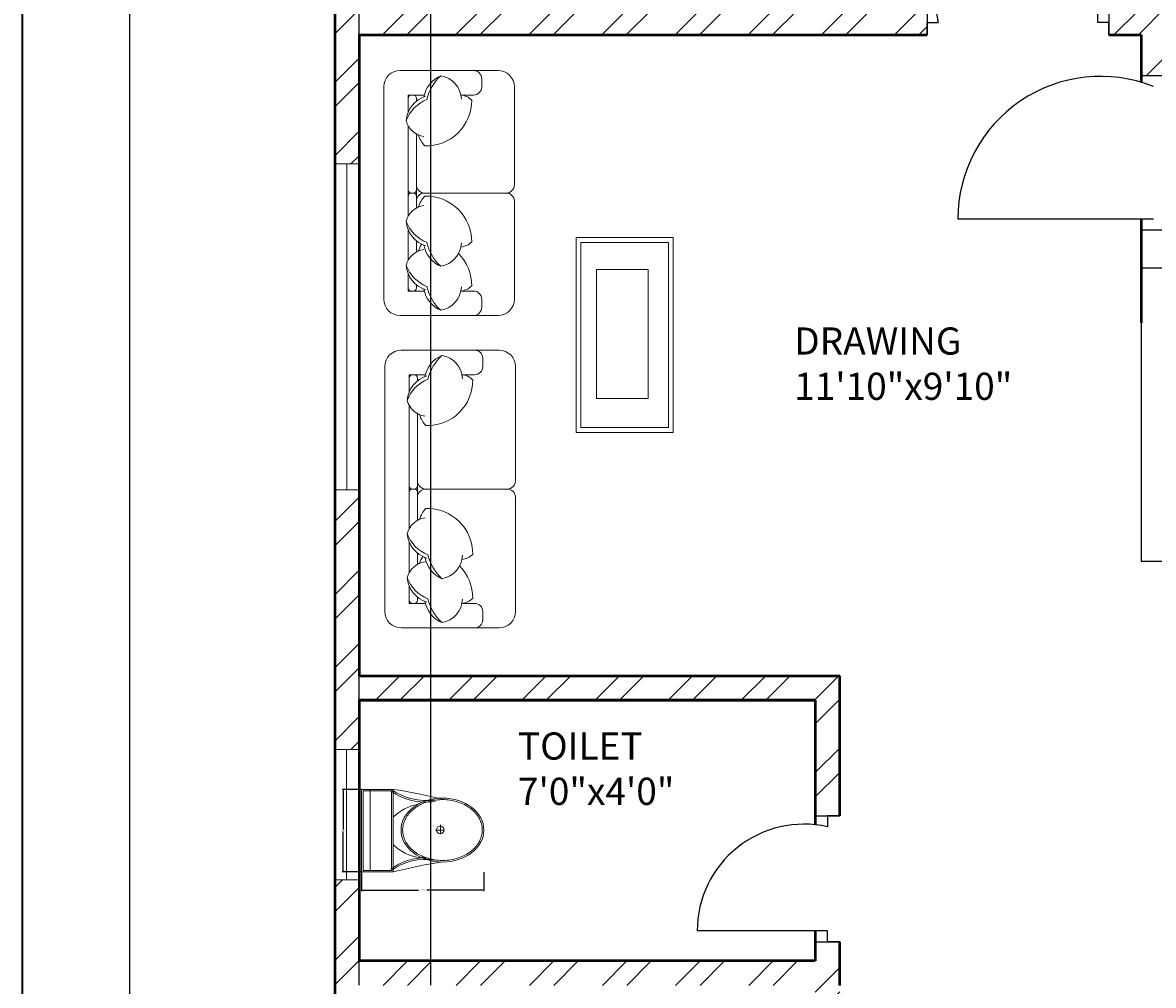
# Model space of a CAD drawing. Units: inches. Extents: x 2129 to 2642, y 1542 to 2414.
# Tile 5 of 9: x 2129 to 2338, y 2007 to 2184. Entities that reach past the tile are written whole.
import ezdxf

# ---------------------------------------------------------------- set-up
doc = ezdxf.new("R2010")
doc.units = ezdxf.units.IN
for name, color, linetype, lineweight in [('A-ANNO-DIMS', 2, 'Continuous', 18), ('A-ANNO-TTLB', 7, 'Continuous', 35), ('A-AREA-IDEN', 7, 'Continuous', 18), ('A-DOOR', 3, 'Continuous', 25), ('A-FLOR-EVTR', 141, 'Continuous', 25), ('A-FLOR-FIXT', 9, 'Continuous', 18), ('A-FURN', 8, 'Continuous', 18), ('A-GLAZ', 4, 'Continuous', 18), ('A-WALL', 7, 'Continuous', 50), ('A-WALL-PATT', 252, 'Continuous', 13)]:
    doc.layers.add(name, color=color, linetype=linetype, lineweight=lineweight)
doc.styles.get("Standard").update_dxf_attribs({"font": 'arial.ttf'})
doc.dimstyles.get("Standard").update_dxf_attribs({"dimtxt": 0.18, "dimasz": 0.18, "dimexe": 0.18, "dimexo": 0.0625, "dimgap": 0.09, "dimtad": 0, "dimtih": 1, "dimtoh": 1, "dimdec": 4, "dimzin": 0, "dimdsep": 46, "dimtxsty": 'Standard', "dimcen": 0.09, "dimadec": 0, "dimazin": 0, "dimtfac": 1, "dimtdec": 4, "dimtofl": 0, "dimtmove": 0, "dimatfit": 3, "dimfxl": 1, "dimtolj": 1, "dimtzin": 0, "dimarcsym": 0})

# ---------------------------------------------------------------- blocks, each defined once
blk = doc.blocks.new('A$C31115884')
for p, q in [((257.5, 466.4), (257.5, 523.2)), ((283.1, 497.7), (223.4, 497.7)), ((0, 200), (0, 0)), ((520, 200), (0, 200)), ((10, 190), (10, 10)), ((510, 190), (10, 190)), ((510, 10), (510, 190)), ((520, 0), (520, 200)), ((510, 54.5), (0, 54.5)), ((10, 10), (510, 10)), ((0, 0), (520, 0))]:
    blk.add_line(p, q)
blk.add_circle((255.6, 496.4), 23.6)
for centre, radius, start, end in [((2777.7, -204.6), 2807, 165.4549, 171.71327), ((3237, 905), 2807, 188.28673, 194.5451), ((-294.5, 403.3), 364.7, 324.20913, 9.34987), ((-294.5, 403.3), 374.7, 324.20913, 9.34987), ((805.8, 403.3), 364.7, 170.65013, 215.79087), ((139.5, 406.2), 293.5, 315.84364, 2.65635), ((805.8, 403.3), 374.7, 179.20365, 215.79087), ((383.6, 406.2), 293.5, 190.27735, 224.15636)]:
    blk.add_arc(centre, radius, start, end)
blk.add_ellipse((256.2, 509.9), major_axis=(0, -260.7), ratio=0.772727)
blk.add_open_spline([(256.2, 259.2), (263.1, 259.2), (270, 259.7), (287.8, 262.3), (298.7, 265.1), (319.9, 273.1), (330.2, 278.4), (350.1, 291.1), (359.7, 298.7), (377.7, 315.9), (386.2, 325.5), (401.7, 346.6), (408.8, 358.1), (421.3, 382.5), (426.8, 395.5), (435.9, 422.4), (439.5, 436.4), (444.8, 465.1), (446.5, 479.7), (447.9, 509.2), (447.6, 524), (445, 553.3), (442.7, 567.8), (436.3, 596), (432.1, 609.7), (421.9, 636), (416, 648.6), (402.5, 672.1), (395, 683), (378.6, 703), (369.8, 712.1), (351.1, 728), (341.3, 734.8), (320.9, 746.2), (310.4, 750.7), (288.9, 757.3), (278, 759.4), (256, 761), (245, 760.6), (223.1, 757.2), (212.3, 754.3), (191.1, 746.1), (180.8, 740.7), (160.9, 727.8), (151.4, 720.1), (133.5, 702.7), (125.1, 693), (109.6, 671.7), (102.6, 660.2), (90.2, 635.7), (84.9, 622.7), (76, 595.6), (72.4, 581.6), (67.2, 552.9), (65.6, 538.2), (64.4, 508.8), (64.8, 494), (67.5, 464.7), (69.9, 450.2), (76.6, 422), (80.8, 408.3), (91.1, 382.2), (97.2, 369.7), (110.8, 346.3), (118.4, 335.4), (134.8, 315.6), (143.7, 306.7), (162.4, 290.9), (172.3, 284.2), (192.8, 273), (203.3, 268.6), (224.8, 262.2), (235.8, 260.2), (249.9, 259.3), (253, 259.2), (256.2, 259.2)], degree=3, knots=[0, 0, 0, 0, 0.110105, 0.110105, 0.285049, 0.285049, 0.459994, 0.459994, 0.634938, 0.634938, 0.809882, 0.809882, 0.984827, 0.984827, 1.159771, 1.159771, 1.334715, 1.334715, 1.50966, 1.50966, 1.684604, 1.684604, 1.859549, 1.859549, 2.034493, 2.034493, 2.209437, 2.209437, 2.384382, 2.384382, 2.559326, 2.559326, 2.73427, 2.73427, 2.909215, 2.909215, 3.084159, 3.084159, 3.259103, 3.259103, 3.434048, 3.434048, 3.608992, 3.608992, 3.783936, 3.783936, 3.958881, 3.958881, 4.133825, 4.133825, 4.30877, 4.30877, 4.483714, 4.483714, 4.658658, 4.658658, 4.833603, 4.833603, 5.008547, 5.008547, 5.183491, 5.183491, 5.358436, 5.358436, 5.53338, 5.53338, 5.708324, 5.708324, 5.883269, 5.883269, 6.058213, 6.058213, 6.233158, 6.233158, 6.283185, 6.283185, 6.283185, 6.283185])
blk = doc.blocks.new('TABLE-COFFEE')
for points in [[(0, 35.92), (17.84, 35.92), (17.84, 0), (0, 0)], [(0.86, 34.99), (17.01, 34.99), (17.01, 0.93), (0.86, 0.93)], [(3.74, 30.05), (13.25, 30.05), (13.25, 6.3), (3.74, 6.3)]]:
    blk.add_lwpolyline(points, close=True)
blk = doc.blocks.new('WIN-60-B')
for p, q in [((4.5, 60), (0, 60)), ((0, 60), (2.25, 60)), ((2.25, 60), (2.25, 0)), ((2.25, 0), (0, 0)), ((0, 0), (4.5, 0))]:
    blk.add_line(p, q)
blk = doc.blocks.new('*D20')
at = {"layer": 'A-ANNO-DIMS', "color": 0, "lineweight": -2, "transparency": 16777216}
for p, q in [((2191.83, 2028.04), (2191.83, 2024.55)), ((2214.37, 2028.04), (2214.37, 2024.55)), ((2192.01, 2024.73), (2202.33, 2024.73)), ((2214.19, 2024.73), (2203.88, 2024.73))]:
    blk.add_line(p, q, dxfattribs=at)
at = {"layer": 'A-ANNO-DIMS', "color": 0, "transparency": 16777216}
for points in [[(2192.01, 2024.76), (2192.01, 2024.7), (2191.83, 2024.73)], [(2214.19, 2024.76), (2214.19, 2024.7), (2214.37, 2024.73)]]:
    blk.add_solid(points, dxfattribs=at)
at = {"layer": 'Defpoints', "color": 0, "transparency": 16777216}
for p in [(2191.83, 2028.11), (2214.37, 2028.11), (2214.37, 2024.73)]:
    blk.add_point(p, dxfattribs=at)
at = {"layer": 'A-ANNO-DIMS', "color": 0, "transparency": 16777216, "insert": (2203.1, 2024.73), "char_height": 0.18, "attachment_point": 5}
blk.add_mtext('\\A1;WC 23 TYP.', dxfattribs=at)
blk = doc.blocks.new('*D21')
at = {"layer": 'A-ANNO-DIMS', "color": 0, "lineweight": -2, "transparency": 16777216}
for p, q in [((2191.77, 2043.31), (2188.27, 2043.31)), ((2188.45, 2043.13), (2188.45, 2035.89)), ((2188.45, 2028.29), (2188.45, 2035.53)), ((2191.77, 2028.11), (2188.27, 2028.11))]:
    blk.add_line(p, q, dxfattribs=at)
at = {"layer": 'A-ANNO-DIMS', "color": 0, "transparency": 16777216}
for points in [[(2188.42, 2043.13), (2188.48, 2043.13), (2188.45, 2043.31)], [(2188.42, 2028.29), (2188.48, 2028.29), (2188.45, 2028.11)]]:
    blk.add_solid(points, dxfattribs=at)
at = {"layer": 'Defpoints', "color": 0, "transparency": 16777216}
for p in [(2191.83, 2043.31), (2188.45, 2028.11), (2191.83, 2028.11)]:
    blk.add_point(p, dxfattribs=at)
at = {"layer": 'A-ANNO-DIMS', "color": 0, "transparency": 16777216, "insert": (2188.45, 2035.71), "char_height": 0.18, "attachment_point": 5}
blk.add_mtext('\\A1;15 TYP.', dxfattribs=at)
blk = doc.blocks.new('*D35')
at = {"layer": 'A-ANNO-DIMS', "color": 0, "lineweight": -2, "transparency": 16777216}
for p, q in [((2186.84, 2340.22), (2148.97, 2340.22)), ((2149.15, 2340.04), (2149.15, 2003.15)), ((2149.15, 1665.9), (2149.15, 2002.79)), ((2186.84, 1665.72), (2148.97, 1665.72))]:
    blk.add_line(p, q, dxfattribs=at)
at = {"layer": 'A-ANNO-DIMS', "color": 0, "transparency": 16777216}
for points in [[(2149.12, 2340.04), (2149.18, 2340.04), (2149.15, 2340.22)], [(2149.12, 1665.9), (2149.18, 1665.9), (2149.15, 1665.72)]]:
    blk.add_solid(points, dxfattribs=at)
at = {"layer": 'Defpoints', "color": 0, "transparency": 16777216}
for p in [(2149.15, 2340.22), (2186.9, 2340.22), (2186.9, 1665.72)]:
    blk.add_point(p, dxfattribs=at)
at = {"layer": 'A-ANNO-DIMS', "color": 0, "transparency": 16777216, "insert": (2149.15, 2002.97), "char_height": 0.18, "attachment_point": 5}
blk.add_mtext('\\A1;674.5', dxfattribs=at)
blk = doc.blocks.new('*D48')
at = {"layer": 'A-ANNO-DIMS', "color": 0, "lineweight": -2, "transparency": 16777216}
for p, q in [((2191.4, 2007.28), (2191.4, 2378.15)), ((2191.58, 2377.97), (2197.54, 2377.97)), ((2204.41, 2377.97), (2198.45, 2377.97)), ((2204.59, 2007.28), (2204.59, 2378.15))]:
    blk.add_line(p, q, dxfattribs=at)
at = {"layer": 'A-ANNO-DIMS', "color": 0, "transparency": 16777216}
for points in [[(2191.58, 2378), (2191.58, 2377.94), (2191.4, 2377.97)], [(2204.41, 2378), (2204.41, 2377.94), (2204.59, 2377.97)]]:
    blk.add_solid(points, dxfattribs=at)
at = {"layer": 'Defpoints', "color": 0, "transparency": 16777216}
for p in [(2204.59, 2377.97), (2191.4, 2007.22), (2204.59, 2007.22)]:
    blk.add_point(p, dxfattribs=at)
at = {"layer": 'A-ANNO-DIMS', "color": 0, "transparency": 16777216, "insert": (2198, 2377.97), "char_height": 0.18, "attachment_point": 5}
blk.add_mtext('\\A1;13.186', dxfattribs=at)

msp = doc.modelspace()

# ---------------------------------------------------------------- hatches: boundary and pattern name
at = {"layer": 'A-WALL-PATT'}
h = msp.add_hatch(dxfattribs=at)
h.set_pattern_fill('ANSI32', color=256)
h.paths.add_polyline_path([(2306.2606, 2305.9717), (2306.2606, 2308.2217), (2276.3515, 2308.2217), (2276.3515, 2303.7217), (2306.2606, 2303.7217)])
h.paths.add_polyline_path([(2216.3515, 2305.9717), (2216.3515, 2308.2217), (2186.9043, 2308.2217), (2186.9043, 2278.1696), (2191.4043, 2278.1696), (2191.4043, 2303.7217), (2216.3515, 2303.7217)])
h.paths.add_polyline_path([(2339.9043, 2335.7217), (2362.1938, 2335.7217), (2362.1938, 2340.2217), (2335.4043, 2340.2217), (2335.4043, 2308.2217), (2329.3487, 2308.2217), (2329.3487, 2305.9717), (2329.3487, 2303.7217), (2335.4043, 2303.7217), (2335.4043, 2186.7217), (2329.4345, 2186.7217), (2329.4345, 2182.2217), (2335.4043, 2182.2217), (2335.4043, 2174.7178), (2339.9043, 2174.7178), (2339.9043, 2182.2217), (2339.9043, 2303.7217)])
h.paths.add_polyline_path([(2440.4043, 2340.2217), (2411.654, 2340.2217), (2411.654, 2335.7217), (2435.9043, 2335.7217), (2435.9043, 2303.7217), (2435.9043, 2182.2217), (2435.9043, 2174.1935), (2438.1543, 2174.1935), (2440.4043, 2174.1935), (2440.4043, 2182.2217), (2444.653, 2182.2217), (2444.653, 2184.4717), (2444.653, 2186.7217), (2440.4043, 2186.7217), (2440.4043, 2303.7217), (2445.8547, 2303.7217), (2445.8547, 2308.2217), (2440.4043, 2308.2217)])
h.paths.add_polyline_path([(2498.2381, 2308.2217), (2470.3901, 2308.2217), (2470.3901, 2303.7217), (2498.2381, 2303.7217), (2498.2381, 2305.9717)])
h.paths.add_polyline_path([(2588.9043, 2308.2217), (2586.9043, 2308.2217), (2558.2381, 2308.2217), (2558.2381, 2303.7217), (2584.4043, 2303.7217), (2584.4043, 2279.1087), (2588.9043, 2279.1087)])
h.paths.add_polyline_path([(2588.9043, 2219.1087), (2584.4043, 2219.1087), (2584.4043, 2186.7217), (2478.0667, 2186.7217), (2478.0667, 2182.2217), (2584.4043, 2182.2217), (2584.4043, 2157.7883), (2588.9043, 2157.7883)])
h.paths.add_polyline_path([(2588.9043, 2097.7883), (2584.6063, 2097.7883), (2584.6063, 2075.5462, -0.09241561), (2584.4043, 2074.4627), (2584.4043, 2064.2217), (2495.9043, 2064.2217), (2495.9043, 2040.4611), (2500.4043, 2040.4611), (2500.4043, 2059.7217), (2584.4043, 2059.7217), (2584.4043, 2052.2164), (2588.9043, 2052.2164)])
h.paths.add_polyline_path([(2588.9043, 2028.2164), (2584.4043, 2028.2164), (2584.4043, 2011.7217), (2500.4043, 2011.7217), (2500.4043, 2015.243), (2498.1543, 2015.243), (2495.9043, 2015.243), (2495.9043, 2007.2217), (2495.9043, 2003.7597), (2500.4043, 2003.7597), (2500.4043, 2007.2217), (2584.4043, 2007.2217), (2584.4043, 1992.1997), (2588.9043, 1992.1997)])
h.paths.add_polyline_path([(2588.9043, 1956.1997), (2584.4043, 1956.1997), (2584.4043, 1941.2217), (2500.4043, 1941.2217), (2500.4043, 1985.1493), (2498.1543, 1985.1493), (2495.9043, 1985.1493), (2495.9043, 1941.2217), (2435.9043, 1941.2217), (2435.9043, 1930.3963), (2440.4043, 1930.3963), (2440.4043, 1936.7217), (2584.4043, 1936.7217), (2584.4043, 1909.8406), (2588.9043, 1909.8406)])
h.paths.add_polyline_path([(2588.9043, 1849.8406), (2584.4043, 1849.8406), (2584.4043, 1801.3526), (2588.9043, 1801.3526)])
h.paths.add_polyline_path([(2584.4043, 1828.7217), (2495.9043, 1828.7217), (2440.4043, 1828.7217), (2440.4043, 1905.2159), (2438.1543, 1905.2159), (2435.9043, 1905.2159), (2435.9043, 1828.7217), (2428.9101, 1828.7217), (2428.9101, 1824.2217), (2584.4043, 1824.2217)])
h.paths.add_polyline_path([(2588.9043, 1741.3526), (2584.4043, 1741.3526), (2584.4043, 1704.2217), (2468.3173, 1704.2217), (2468.3173, 1701.9717), (2468.3173, 1699.7217), (2588.9043, 1699.7217)])
h.paths.add_polyline_path([(2442.4043, 1761.7217), (2435.0216, 1761.7217), (2435.0216, 1757.2217), (2437.9043, 1757.2217), (2437.9043, 1665.7217), (2442.4043, 1665.7217), (2442.4043, 1667.7217), (2442.4043, 1699.7217), (2446.6907, 1699.7217), (2446.6907, 1701.9717), (2446.6907, 1704.2217), (2442.4043, 1704.2217)])
h.paths.add_polyline_path([(2390.4043, 1757.2217), (2410.8996, 1757.2217), (2410.8996, 1761.7217), (2360.1741, 1761.7217), (2360.1741, 1759.4717), (2360.1741, 1757.2217), (2385.9043, 1757.2217), (2385.9043, 1674.8326), (2390.4043, 1674.8326)])
h.paths.add_polyline_path([(2337.9043, 1757.2217), (2340.3592, 1757.2217), (2340.3592, 1759.4717), (2340.3592, 1761.7217), (2333.4043, 1761.7217), (2333.4043, 1704.2217), (2327.381, 1704.2217), (2327.381, 1701.9717), (2327.381, 1699.7217), (2333.4043, 1699.7217), (2333.4043, 1665.7217), (2337.9043, 1665.7217)])
h.paths.add_polyline_path([(2191.4043, 1743.4804), (2186.9043, 1743.4804), (2186.9043, 1699.7217), (2188.9043, 1699.7217), (2191.4043, 1699.7217), (2306.5617, 1699.7217), (2306.5617, 1704.2217), (2191.4043, 1704.2217)])
h.paths.add_polyline_path([(2191.4043, 1859.8992), (2186.9043, 1859.8992), (2186.9043, 1803.4804), (2189.1543, 1803.4804), (2191.4043, 1803.4804)])
h.paths.add_polyline_path([(2352.5445, 1828.7217), (2191.4043, 1828.7217), (2191.4043, 1824.2217), (2333.4043, 1824.2217), (2352.5445, 1824.2217), (2352.5445, 1826.4717)])
h.paths.add_polyline_path([(2390.4043, 2085.328), (2385.9043, 2085.328), (2385.9043, 1828.7217), (2381.9668, 1828.7217), (2381.9668, 1826.4717), (2381.9668, 1824.2217), (2385.9043, 1824.2217), (2385.9043, 1761.7217), (2390.4043, 1761.7217), (2390.4043, 1824.2217), (2394.1868, 1824.2217), (2394.1868, 1827.6339), (2394.1868, 1828.7217), (2390.4043, 1828.7217)])
h.paths.add_polyline_path([(2339.9043, 1941.2217), (2335.4043, 1941.2217), (2279.9043, 1941.2217), (2279.9043, 1981.3432), (2277.6543, 1981.3432), (2275.4043, 1981.3432), (2275.4043, 1941.2217), (2191.4043, 1941.2217), (2191.4043, 1958.1079), (2186.9043, 1958.1079), (2186.9043, 1919.8992), (2189.1543, 1919.8992), (2191.4043, 1919.8992), (2191.4043, 1936.7217), (2279.9043, 1936.7217), (2335.4043, 1936.7217), (2335.4043, 1931.1382), (2339.9043, 1931.1382)])
h.paths.add_polyline_path([(2339.9043, 1902.7544), (2337.6543, 1902.7544), (2335.4043, 1902.7544), (2335.4043, 1828.7217), (2339.9043, 1828.7217)])
h.paths.add_polyline_path([(2279.9043, 2015.263), (2277.6543, 2015.263), (2275.4043, 2015.263), (2275.4043, 2011.7217), (2191.4043, 2011.7217), (2191.4043, 2026.6781), (2186.9043, 2026.6781), (2186.9043, 1994.1079), (2189.1543, 1994.1079), (2191.4043, 1994.1079), (2191.4043, 2007.2217), (2275.4043, 2007.2217), (2275.4043, 2003.2288), (2279.9043, 2003.2288), (2279.9043, 2007.2217)])
h.paths.add_polyline_path([(2296.0216, 2186.7217), (2191.4043, 2186.7217), (2191.4043, 2218.1696), (2186.9043, 2218.1696), (2186.9043, 2158.4509), (2191.4043, 2158.4509), (2191.4043, 2182.2217), (2296.0216, 2182.2217), (2296.0216, 2184.4717)])
h.paths.add_polyline_path([(2191.4043, 2098.4509), (2189.1543, 2098.4509), (2186.9043, 2098.4509), (2186.9043, 2050.6781), (2189.0487, 2050.6781), (2191.4043, 2050.6781), (2191.4043, 2059.7217), (2275.4043, 2059.7217), (2275.4043, 2038.4133), (2279.9043, 2038.4133), (2279.9043, 2064.2217), (2191.4043, 2064.2217)])
h.paths.add_polyline_path([(2268.3923, 1605.9386), (2516.3159, 1605.9386), (2516.3159, 1643.0314), (2268.3923, 1643.0314)], flags=9)
h.paths.add_polyline_path([(2399.6079, 1710.4489), (2428.8405, 1710.4489), (2428.8405, 1729.1062), (2399.6079, 1729.1062)], flags=9)
h.paths.add_polyline_path([(2342.1483, 1708.9956), (2371.3809, 1708.9956), (2371.3809, 1727.653), (2342.1483, 1727.653)], flags=9)
h.paths.add_polyline_path([(2200.7404, 1677.2519), (2282.3059, 1677.2519), (2282.3059, 1687.5555), (2200.7404, 1687.5555)], flags=9)
h.paths.add_polyline_path([(2209.8153, 1704.7448), (2250.627, 1704.7448), (2250.627, 1723.4021), (2209.8153, 1723.4021)], flags=25)
h.paths.add_polyline_path([(2213.9996, 1911.284), (2252.84, 1911.284), (2252.84, 1929.9413), (2213.9996, 1929.9413)], flags=9)
h.paths.add_polyline_path([(2210.8865, 1962.0987), (2244.0447, 1962.0987), (2244.0447, 1980.7561), (2210.8865, 1980.7561)], flags=25)
h.paths.add_polyline_path([(2219.0745, 2037.6131), (2248.2321, 2037.6131), (2248.2321, 2056.2705), (2219.0745, 2056.2705)], flags=9)
h.paths.add_polyline_path([(2379.9702, 2099.0686), (2409.3767, 2099.0686), (2409.3767, 2117.7259), (2379.9702, 2117.7259)], flags=9)
h.paths.add_polyline_path([(2375.9312, 2160.3752), (2405.3173, 2160.3752), (2405.3173, 2179.0325), (2375.9312, 2179.0325)], flags=9)
h.paths.add_polyline_path([(2269.5058, 2112.1824), (2310.3175, 2112.1824), (2310.3175, 2130.8397), (2269.5058, 2130.8397)], flags=9)
h.paths.add_polyline_path([(2209.6567, 2193.667), (2248.4971, 2193.667), (2248.4971, 2212.3243), (2209.6567, 2212.3243)], flags=25)
h.paths.add_polyline_path([(2491.6289, 1675.447), (2573.1944, 1675.447), (2573.1944, 1685.7506), (2491.6289, 1685.7506)], flags=9)
h.paths.add_polyline_path([(2492.0585, 1710.4489), (2530.8989, 1710.4489), (2530.8989, 1729.1062), (2492.0585, 1729.1062)], flags=25)
h.paths.add_polyline_path([(2495.6634, 1908.8646), (2534.5038, 1908.8646), (2534.5038, 1927.522), (2495.6634, 1927.522)], flags=9)
h.paths.add_polyline_path([(2516.7779, 1955.9942), (2549.9362, 1955.9942), (2549.9362, 1974.6516), (2516.7779, 1974.6516)], flags=25)
h.paths.add_polyline_path([(2509.7444, 2034.6896), (2538.902, 2034.6896), (2538.902, 2053.347), (2509.7444, 2053.347)], flags=9)
h.paths.add_polyline_path([(2467.8454, 2111.9593), (2508.6571, 2111.9593), (2508.6571, 2130.6167), (2467.8454, 2130.6167)], flags=9)
h.paths.add_polyline_path([(2528.5267, 2189.1742), (2567.3671, 2189.1742), (2567.3671, 2207.8316), (2528.5267, 2207.8316)], flags=25)
h.paths.add_polyline_path([(2483.7603, 2319.9841), (2557.5563, 2319.9841), (2557.5563, 2330.2877), (2483.7603, 2330.2877)], flags=9)
h.paths.add_polyline_path([(2204.078, 2317.0445), (2277.874, 2317.0445), (2277.874, 2327.3481), (2204.078, 2327.3481)], flags=9)

# ---------------------------------------------------------------- linework, layer by layer
at = {"layer": 'A-ANNO-TTLB'}
msp.add_lwpolyline([(2129.4387, 2413.7704), (2642.2731, 2413.7704), (2642.2731, 1542.3836), (2129.4387, 1542.3836)], close=True, dxfattribs=at)
at = {"layer": 'A-DOOR'}
for p, q in [((2327.4345, 2184.4717), (2327.4345, 2220.4717)), ((2296.0216, 2186.7217), (2296.0216, 2182.2217)), ((2329.4345, 2186.7217), (2329.4345, 2182.2217)), ((2296.0216, 2182.2217), (2296.0216, 2184.4717)), ((2296.0216, 2184.4717), (2298.0216, 2184.4717)), ((2329.4345, 2184.4717), (2327.4345, 2184.4717)), ((2329.4345, 2182.2217), (2329.4345, 2184.4717)), ((2335.4043, 2174.7178), (2339.9043, 2174.7178)), ((2337.6543, 2148.2947), (2301.6543, 2148.2947)), ((2335.4043, 2146.2947), (2339.9043, 2146.2947)), ((2275.4043, 2038.4133), (2279.9043, 2038.4133)), ((2279.9043, 2038.4133), (2277.6543, 2038.4133)), ((2277.6543, 2038.4133), (2277.6543, 2036.4133)), ((2277.6543, 2017.263), (2253.6543, 2017.263)), ((2277.6543, 2015.263), (2277.6543, 2017.263)), ((2275.4043, 2015.263), (2279.9043, 2015.263)), ((2279.9043, 2015.263), (2277.6543, 2015.263))]:
    msp.add_line(p, q, dxfattribs=at)
for centre, radius, start, end in [((2327.4345, 2190.4562), 30.0155, 90, 191.500693), ((2327.9389, 2148.2947), 26.2846, 68.307494, 180), ((2273.2947, 2017.263), 19.6403, 77.174899, 180)]:
    msp.add_arc(centre, radius, start, end, dxfattribs=at)
at = {"layer": 'A-FLOR-EVTR'}
for p, q in [((2335.4043, 2139.328), (2440.4043, 2139.328)), ((2335.4043, 2139.328), (2335.4043, 2085.328)), ((2335.4043, 2085.328), (2440.4043, 2085.328))]:
    msp.add_line(p, q, dxfattribs=at)
at = {"layer": 'A-FURN', "ltscale": 0.03}
for points in [[(2219.9866, 2154.6047, -0.41421356), (2218.4832, 2153.1013, -0.41421356), (2219.9866, 2151.5979), (2219.9866, 2133.5569, -0.41421356), (2216.9798, 2130.5501), (2198.9389, 2130.5501, -0.41421356), (2195.932, 2133.5569), (2195.932, 2172.6456, -0.41421356), (2198.9389, 2175.6525), (2216.9798, 2175.6525, -0.41421356), (2219.9866, 2172.6456), (2219.9866, 2154.6047, -0.41421356), (2218.4832, 2153.1013, -0.41421356), (2219.9866, 2151.5979)], [(2220.1886, 2100.1052, -0.41421356), (2218.6852, 2098.6018, -0.41421356), (2220.1886, 2097.0984), (2220.1886, 2076.0506, -0.41421356), (2217.1818, 2073.0438), (2199.1408, 2073.0438, -0.41421356), (2196.134, 2076.0506), (2196.134, 2121.153, -0.41421356), (2199.1408, 2124.1598), (2217.1818, 2124.1598, -0.41421356), (2220.1886, 2121.153), (2220.1886, 2100.1052, -0.41421356), (2218.6852, 2098.6018, -0.41421356), (2220.1886, 2097.0984)]]:
    msp.add_lwpolyline(points, format="xyb", dxfattribs=at)
at = {"layer": 'A-FURN'}
for points in [[(2206.4417, 2174.6956, 0.14772988), (2203.8579, 2170.3016, 0.21334276), (2200.0684, 2166.4245, 0.17866181)], [(2210.2312, 2170.3877, 0.35677236), (2206.4417, 2174.6956, 0.24954205), (2203.3188, 2170.7923, -9.61688035)], [(2212.4696, 2175.6525, -0.41421356), (2213.973, 2174.149), (2213.973, 2172.6456, -0.41421356), (2212.4696, 2171.1422), (2210.1402, 2171.1422)], [(2203.652, 2170.9086, 0.30666349), (2200.0684, 2166.4245, 0.30632997), (2203.3412, 2163.4951, -0.87284716)], [(2201.9457, 2169.9949), (2201.9457, 2170.5409, 0.41421356), (2201.3443, 2171.1422), (2201.0436, 2171.1422, 0.41421356), (2200.4423, 2170.5409)], [(2200.4423, 2170.5409), (2200.4423, 2167.9795, 0.41421356)], [(2210.1396, 2171.1455, -0.16554063), (2212.126, 2170.2154, -0.42598917), (2203.5134, 2161.772, -0.12152332), (2202.3263, 2163.7763, 7.11546429)], [(2200.4423, 2165.4783), (2200.4423, 2153.7026, 0.41421356), (2201.0436, 2153.1013), (2201.3443, 2153.1013, 0.41421356), (2201.9457, 2153.7026), (2201.9457, 2163.9645, 0.41421356)], [(2200.4423, 2148.823), (2200.4423, 2152.4999, -0.41421356), (2201.0436, 2153.1013), (2201.3443, 2153.1013, -0.41421356), (2201.9457, 2152.4999), (2201.9457, 2150.3369, -0.41421356)], [(2201.9457, 2154.6047, 0.41421356), (2203.4491, 2153.1013)], [(2201.9457, 2154.6047, 0.41421356), (2203.4491, 2153.1013), (2218.4832, 2153.1013, 0.41421356)], [(2201.9457, 2151.5979, -0.41421356), (2203.4491, 2153.1013)], [(2201.9457, 2151.5979, -0.41421356), (2203.4491, 2153.1013), (2218.4832, 2153.1013, -0.41421356)], [(2210.1396, 2143.1559, 0.16554063), (2212.126, 2144.0859, 0.42598917), (2203.5134, 2152.5294, 0.12152332), (2202.3263, 2150.5251, -7.11546429)], [(2203.652, 2143.3927, -0.30666349), (2200.0684, 2147.8769, -0.30632997), (2203.3412, 2150.8062, 0.87284716)], [(2206.4417, 2139.6057, -0.14772988), (2203.8579, 2143.9998, -0.21334276), (2200.0684, 2147.8769, -0.17866181)], [(2200.4423, 2140.7242), (2200.4423, 2146.3219, -0.41421356)], [(2203.652, 2135.2939, -0.30666349), (2200.0684, 2139.778, -0.30632997), (2203.3412, 2142.7074, 0.87284716)], [(2201.9457, 2144.3064), (2201.9457, 2142.2381, -0.41421356)], [(2202.9141, 2143.6867, 0.07186538), (2202.3263, 2142.4262, -7.11546429)], [(2210.2312, 2143.9136, -0.35677236), (2206.4417, 2139.6057, -0.24954205), (2203.3188, 2143.5091, 9.61688035)], [(2210.1396, 2135.057, 0.16554063), (2212.126, 2135.9871, 0.20023115), (2209.7067, 2141.9551, 0.12152332)], [(2206.4417, 2131.5069, -0.14772988), (2203.8579, 2135.9009, -0.21334276), (2200.0684, 2139.778, -0.17866181)], [(2200.4423, 2135.6617), (2200.4423, 2138.2231, -0.41421356)], [(2200.4423, 2138.2231), (2200.4423, 2135.0603), (2203.3968, 2135.0603, -0.41421356)], [(2201.9457, 2136.2076), (2201.9457, 2135.6617, -0.41421356), (2201.3443, 2135.0603), (2201.0436, 2135.0603, -0.41421356), (2200.4423, 2135.6617)], [(2210.2312, 2135.8148, -0.35677236), (2206.4417, 2131.5069, -0.24954205), (2203.3188, 2135.4102, 9.61688035)], [(2210.1402, 2135.0603), (2212.4696, 2135.0603, -0.41421356), (2213.973, 2133.5569), (2213.973, 2132.0535, -0.41421356), (2212.4696, 2130.5501)], [(2212.6715, 2124.1598, -0.41421356), (2214.175, 2122.6564), (2214.175, 2121.153, -0.41421356), (2212.6715, 2119.6496), (2210.3422, 2119.6496)], [(2206.6437, 2123.203, 0.14772988), (2204.0599, 2118.8089, 0.21334276), (2200.2704, 2114.9318, 0.17866181)], [(2210.4332, 2118.8951, 0.35677236), (2206.6437, 2123.203, 0.24954205), (2203.5208, 2119.2996, -9.61688035)], [(2202.1477, 2118.5023), (2202.1477, 2119.0482, 0.41421356), (2201.5463, 2119.6496), (2201.2456, 2119.6496, 0.41421356), (2200.6442, 2119.0482)], [(2210.3415, 2119.6528, -0.16554063), (2212.328, 2118.7228, -0.42598917), (2203.7154, 2110.2793, -0.12152332), (2202.5283, 2112.2836, 7.11546429)], [(2203.854, 2119.416, 0.30666349), (2200.2704, 2114.9318, 0.30632997), (2203.5432, 2112.0025, -0.87284716)], [(2200.6442, 2119.0482), (2200.6442, 2116.4868, 0.41421356)], [(2200.6442, 2113.9857), (2200.6442, 2099.2031, 0.41421356), (2201.2456, 2098.6018), (2201.5463, 2098.6018, 0.41421356), (2202.1477, 2099.2031), (2202.1477, 2112.4718, 0.41421356)], [(2202.1477, 2100.1052, 0.41421356), (2203.6511, 2098.6018)], [(2202.1477, 2100.1052, 0.41421356), (2203.6511, 2098.6018), (2218.6852, 2098.6018, 0.41421356)], [(2200.6442, 2091.3167), (2200.6442, 2098.0004, -0.41421356), (2201.2456, 2098.6018), (2201.5463, 2098.6018, -0.41421356), (2202.1477, 2098.0004), (2202.1477, 2092.8306, -0.41421356)], [(2202.1477, 2097.0984, -0.41421356), (2203.6511, 2098.6018)], [(2202.1477, 2097.0984, -0.41421356), (2203.6511, 2098.6018), (2218.6852, 2098.6018, -0.41421356)], [(2210.3415, 2085.6496, 0.16554063), (2212.328, 2086.5796, 0.42598917), (2203.7154, 2095.0231, 0.12152332), (2202.5283, 2093.0188, -7.11546429)], [(2203.854, 2085.8864, -0.30666349), (2200.2704, 2090.3706, -0.30632997), (2203.5432, 2093.2999, 0.87284716)], [(2206.6437, 2082.0994, -0.14772988), (2204.0599, 2086.4935, -0.21334276), (2200.2704, 2090.3706, -0.17866181)], [(2200.6442, 2083.2179), (2200.6442, 2088.8156, -0.41421356)], [(2202.1477, 2086.8001), (2202.1477, 2084.7317, -0.41421356)], [(2210.4332, 2086.4073, -0.35677236), (2206.6437, 2082.0994, -0.24954205), (2203.5208, 2086.0027, 9.61688035)], [(2203.854, 2077.7876, -0.30666349), (2200.2704, 2082.2717, -0.30632997), (2203.5432, 2085.2011, 0.87284716)], [(2203.1161, 2086.1804, 0.07186538), (2202.5283, 2084.9199, -7.11546429)], [(2210.3415, 2077.5507, 0.16554063), (2212.328, 2078.4808, 0.20023115), (2209.9087, 2084.4488, 0.12152332)], [(2206.6437, 2074.0006, -0.14772988), (2204.0599, 2078.3946, -0.21334276), (2200.2704, 2082.2717, -0.17866181)], [(2200.6442, 2080.7168), (2200.6442, 2077.554), (2203.5988, 2077.554, -0.41421356)], [(2200.6442, 2078.1554), (2200.6442, 2080.7168, -0.41421356)], [(2202.1477, 2078.7013), (2202.1477, 2078.1554, -0.41421356), (2201.5463, 2077.554), (2201.2456, 2077.554, -0.41421356), (2200.6442, 2078.1554)], [(2210.4332, 2078.3085, -0.35677236), (2206.6437, 2074.0006, -0.24954205), (2203.5208, 2077.9039, 9.61688035)], [(2210.3422, 2077.554), (2212.6715, 2077.554, -0.41421356), (2214.175, 2076.0506), (2214.175, 2074.5472, -0.41421356), (2212.6715, 2073.0438)]]:
    msp.add_lwpolyline(points, format="xyb", dxfattribs=at)
for points in [[(2203.3968, 2171.1422), (2200.4423, 2171.1422), (2200.4423, 2167.9795)], [(2200.4423, 2165.4783), (2200.4423, 2148.823)], [(2200.4423, 2146.3219), (2200.4423, 2140.7242)], [(2203.5988, 2119.6496), (2200.6442, 2119.6496), (2200.6442, 2116.4868)], [(2200.6442, 2113.9857), (2200.6442, 2091.3167)], [(2200.6442, 2088.8156), (2200.6442, 2083.2179)]]:
    msp.add_lwpolyline(points, dxfattribs=at)
for points in [[(2200.4423, 2153.7026), (2200.4423, 2152.4999, -0.41421356), (2201.0436, 2153.1013), (2201.3443, 2153.1013, -0.41421356), (2201.9457, 2152.4999), (2201.9457, 2153.7026, -0.41421356), (2201.3443, 2153.1013), (2201.0436, 2153.1013, -0.41421356)], [(2200.6442, 2099.2031), (2200.6442, 2098.0004, -0.41421356), (2201.2456, 2098.6018), (2201.5463, 2098.6018, -0.41421356), (2202.1477, 2098.0004), (2202.1477, 2099.2031, -0.41421356), (2201.5463, 2098.6018), (2201.2456, 2098.6018, -0.41421356)]]:
    msp.add_lwpolyline(points, format="xyb", close=True, dxfattribs=at)
at = {"layer": 'A-GLAZ'}
for p, q in [((2186.9043, 2050.6781), (2189.0487, 2050.6781)), ((2189.0487, 2050.6781), (2191.4043, 2050.6781)), ((2191.4043, 2050.6781), (2189.0487, 2050.6781)), ((2189.0487, 2050.6781), (2189.0487, 2026.6781)), ((2189.0487, 2026.6781), (2186.9043, 2026.6781)), ((2186.9043, 2026.6781), (2191.4043, 2026.6781))]:
    msp.add_line(p, q, dxfattribs=at)
at = {"layer": 'A-WALL'}
for p, q in [((2186.9043, 2308.2217), (2186.9043, 1699.7217)), ((2191.4043, 2182.2217), (2296.0216, 2182.2217)), ((2191.4043, 2182.2217), (2191.4043, 2064.2217)), ((2191.4043, 2182.2217), (2191.4043, 2064.2217)), ((2329.4345, 2182.2217), (2335.4043, 2182.2217)), ((2335.4043, 2182.2217), (2335.4043, 2173.4968)), ((2335.4043, 2148.2947), (2335.4043, 2129.2217)), ((2191.4043, 2064.2217), (2279.9043, 2064.2217)), ((2279.9043, 2038.4133), (2279.9043, 2064.2217)), ((2191.4043, 2059.7217), (2275.4043, 2059.7217)), ((2275.4043, 2059.7217), (2191.4043, 2059.7217)), ((2191.4043, 2059.7217), (2191.4043, 2011.7217)), ((2275.4043, 2059.7217), (2275.4043, 2036.7897)), ((2275.4043, 2017.263), (2275.4043, 2011.7217)), ((2279.9043, 2007.2217), (2279.9043, 2015.263)), ((2275.4043, 2011.7217), (2191.4043, 2011.7217))]:
    msp.add_line(p, q, dxfattribs=at)

# ---------------------------------------------------------------- block references
at = {"layer": 'A-FLOR-FIXT', "xscale": 0.0292470664339069, "yscale": 0.0292470664339069, "zscale": 0.0292470664339069, "rotation": 270}
msp.add_blockref('A$C31115884', (2191.8333, 2043.3146), dxfattribs=at)
at = {"layer": 'A-FURN'}
msp.add_blockref('TABLE-COFFEE', (2231.375, 2108.98), dxfattribs=at)
at = {"layer": 'A-GLAZ', "rotation": 180}
msp.add_blockref('WIN-60-B', (2191.4047, 2158.4513), dxfattribs=at)

# ---------------------------------------------------------------- texts
at = {"layer": 'A-AREA-IDEN', "char_height": 5, "attachment_point": 1}
for s, width, insert in [('DRAWING\\P11\'10"x9\'10"', 103.806043, (2271.5164, 2128.3517)), ('TOILET\\P7\'0"x4\'0"', 95.342297, (2220.6553, 2053.7858))]:
    msp.add_mtext_dynamic_manual_height_columns(s, width=width, gutter_width=12.5, heights=[0], dxfattribs=dict(at, insert=insert))

# ---------------------------------------------------------------- dimensions: what is measured, and where the dimension line sits
at = {"layer": 'A-ANNO-DIMS'}
dim = msp.add_linear_dim(base=(2204.5902, 2377.9717), p1=(2191.4043, 2007.2217), p2=(2204.5902, 2007.2217), dimstyle='Standard', override={"dimdec": 3, "dimlfac": 1, "dimrnd": 0, "dimzin": 0, "dimdsep": 46, "dimlunit": 2}, dxfattribs=at)
dim.commit()
dim.dimension.update_dxf_attribs({"geometry": '*D48', "text_midpoint": (2197.9973, 2377.9717)})
dim = msp.add_linear_dim(base=(2149.1543, 2340.2217), p1=(2186.9043, 1665.7217), p2=(2186.9043, 2340.2217), angle=90, dimstyle='Standard', override={"dimdec": 1, "dimlfac": 1, "dimrnd": 0, "dimzin": 0, "dimdsep": 46, "dimlunit": 2}, dxfattribs=at)
dim.commit()
dim.dimension.update_dxf_attribs({"geometry": '*D35', "text_midpoint": (2149.1543, 2002.9717)})
dim = msp.add_linear_dim(base=(2188.4528, 2028.1061), p1=(2191.8333, 2043.3146), p2=(2191.8333, 2028.1061), angle=270, text='<> TYP.', dimstyle='Standard', override={"dimdec": 0, "dimlfac": 1, "dimrnd": 0, "dimzin": 0, "dimdsep": 46, "dimlunit": 2}, dxfattribs=at)
dim.commit()
dim.dimension.update_dxf_attribs({"geometry": '*D21', "text_midpoint": (2188.4528, 2035.7104)})
dim = msp.add_linear_dim(base=(2214.3702, 2024.7256), p1=(2191.8333, 2028.1061), p2=(2214.3702, 2028.1061), text='WC <> TYP.', dimstyle='Standard', override={"dimdec": 0, "dimlfac": 1, "dimrnd": 0, "dimzin": 0, "dimdsep": 46, "dimlunit": 2}, dxfattribs=at)
dim.commit()
dim.dimension.update_dxf_attribs({"geometry": '*D20', "text_midpoint": (2203.1018, 2024.7256)})

doc.saveas('drawing.dxf')
